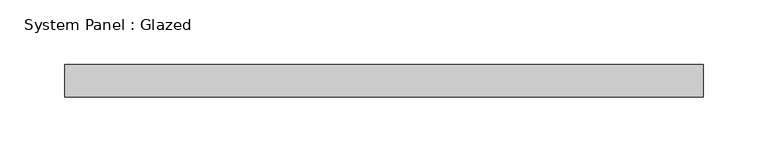
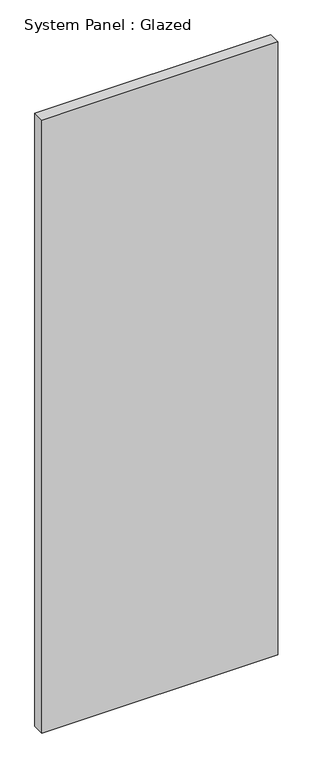
"""IFC4 building model written with IfcOpenShell, lengths in millimetres: plate geometry, System Panel : Glazed."""

from ifc_helpers import new_model, si_unit, origin, origin_with_axes, place, context, project, spatial, polyline, outline, extrude, source, transform, mapped, element, save


def system_panel_glazed_bdb83165(model_context):
    return source(origin(), model_context, "Body", "SweptSolid", [
        extrude(outline(polyline([(247.65, 19.05), (-247.65, 19.05), (-247.65, 44.45), (247.65, 44.45), (247.65, 19.05)])), origin_with_axes(), (0.0, 0.0, 1.0), 1359.8504732),
    ])


if __name__ == "__main__":
    model = new_model("IFC4")
    model_context = context("Model", 3, world=origin())
    ifc_project = project(units=[si_unit("LENGTHUNIT", "METRE", prefix="MILLI")], contexts=[model_context])
    site = spatial("IfcSite", under=ifc_project)
    building = spatial("IfcBuilding", under=site)
    placement = place(None, origin())
    system_panel_glazed_shape = system_panel_glazed_bdb83165(model_context)
    element("IfcPlate", 1, ObjectType="System Panel : Glazed", at=placement, inside=building, context=model_context, shape_type="MappedRepresentation", body=[
        mapped(system_panel_glazed_shape, transform((0.0, 0.0, 0.0), x_axis=(1.0, 0.0, 0.0), y_axis=(0.0, 1.0, 0.0), z_axis=(0.0, 0.0, 1.0))),
    ])
    save(model, "model.ifc")

# Revit data of these elements
# Type "System Panel : Glazed"
#   Construction Type Id = "GSP4R"
#   Analytic Construction = "1/8 in Pilkington single glazing"
#   Visual Light Transmittance = 0.9
#   Solar Heat Gain Coefficient = 0.86
#   Heat Transfer Coefficient (U) = 1.18115 BTU/(h·ft²·°F)
#   Define Thermal Properties by = 1
# Element 1 (IfcPlate, "System Panel : Glazed")
#   Materials on its faces: "Glass"
# Materials
#   "Glass": class "Glass", colour RGB 0 128 192, transparency 0.75, Description = "Soda Lime Glass", Cost = 0
